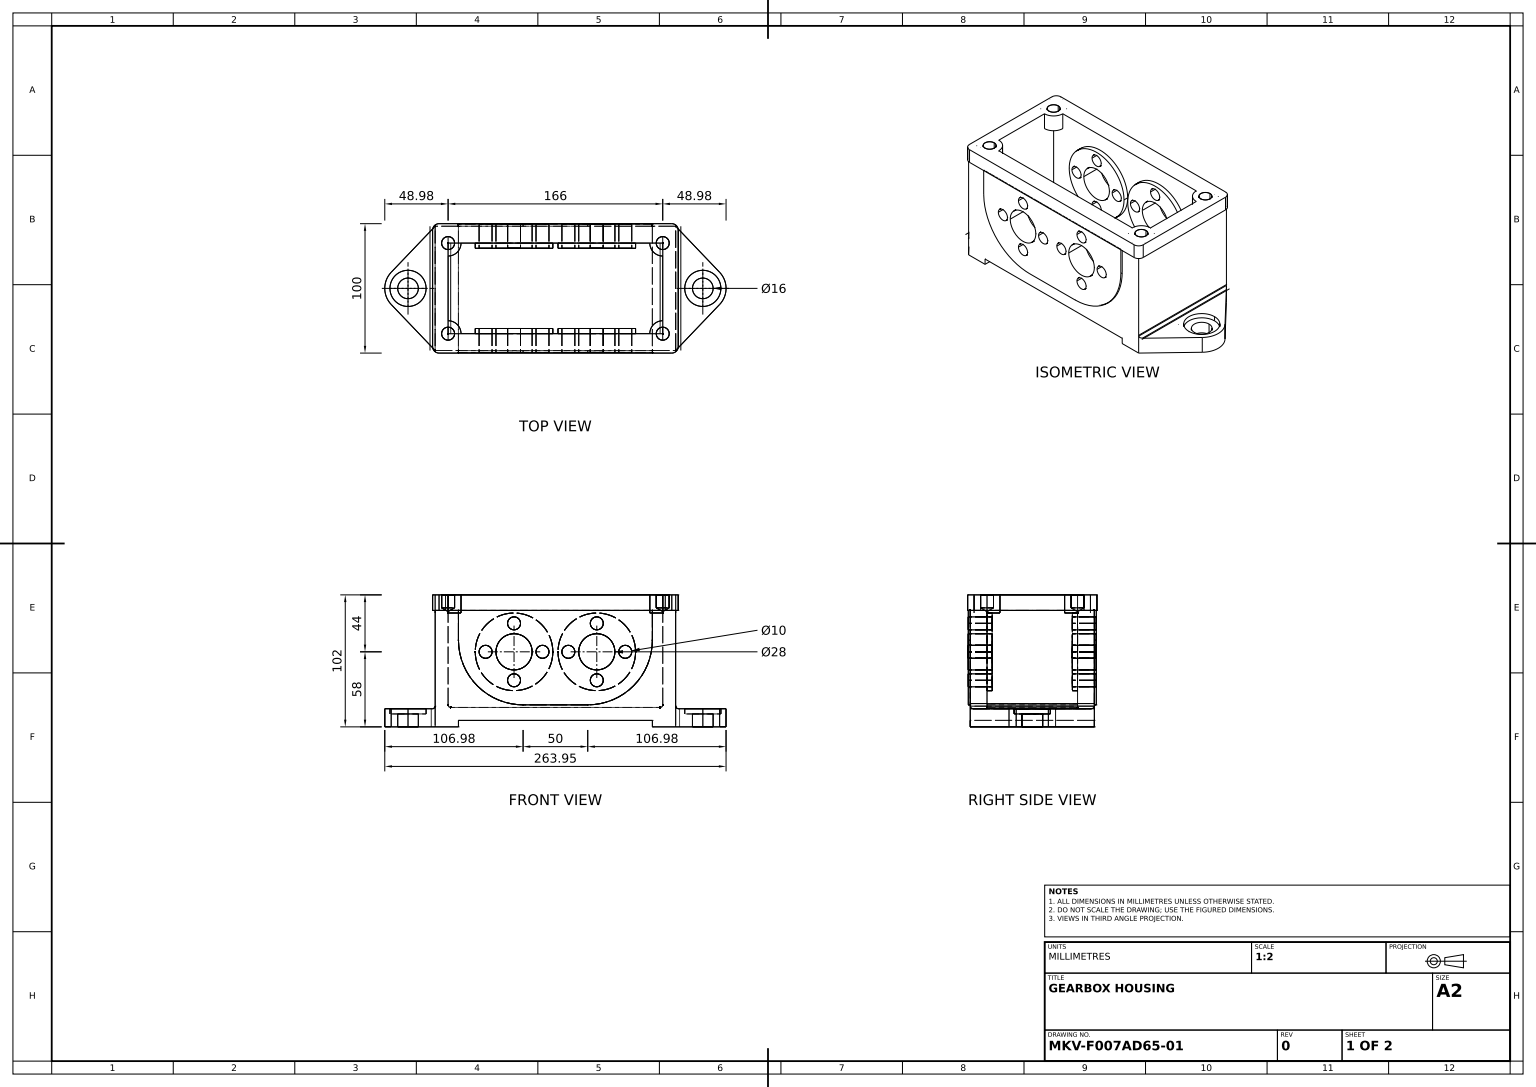
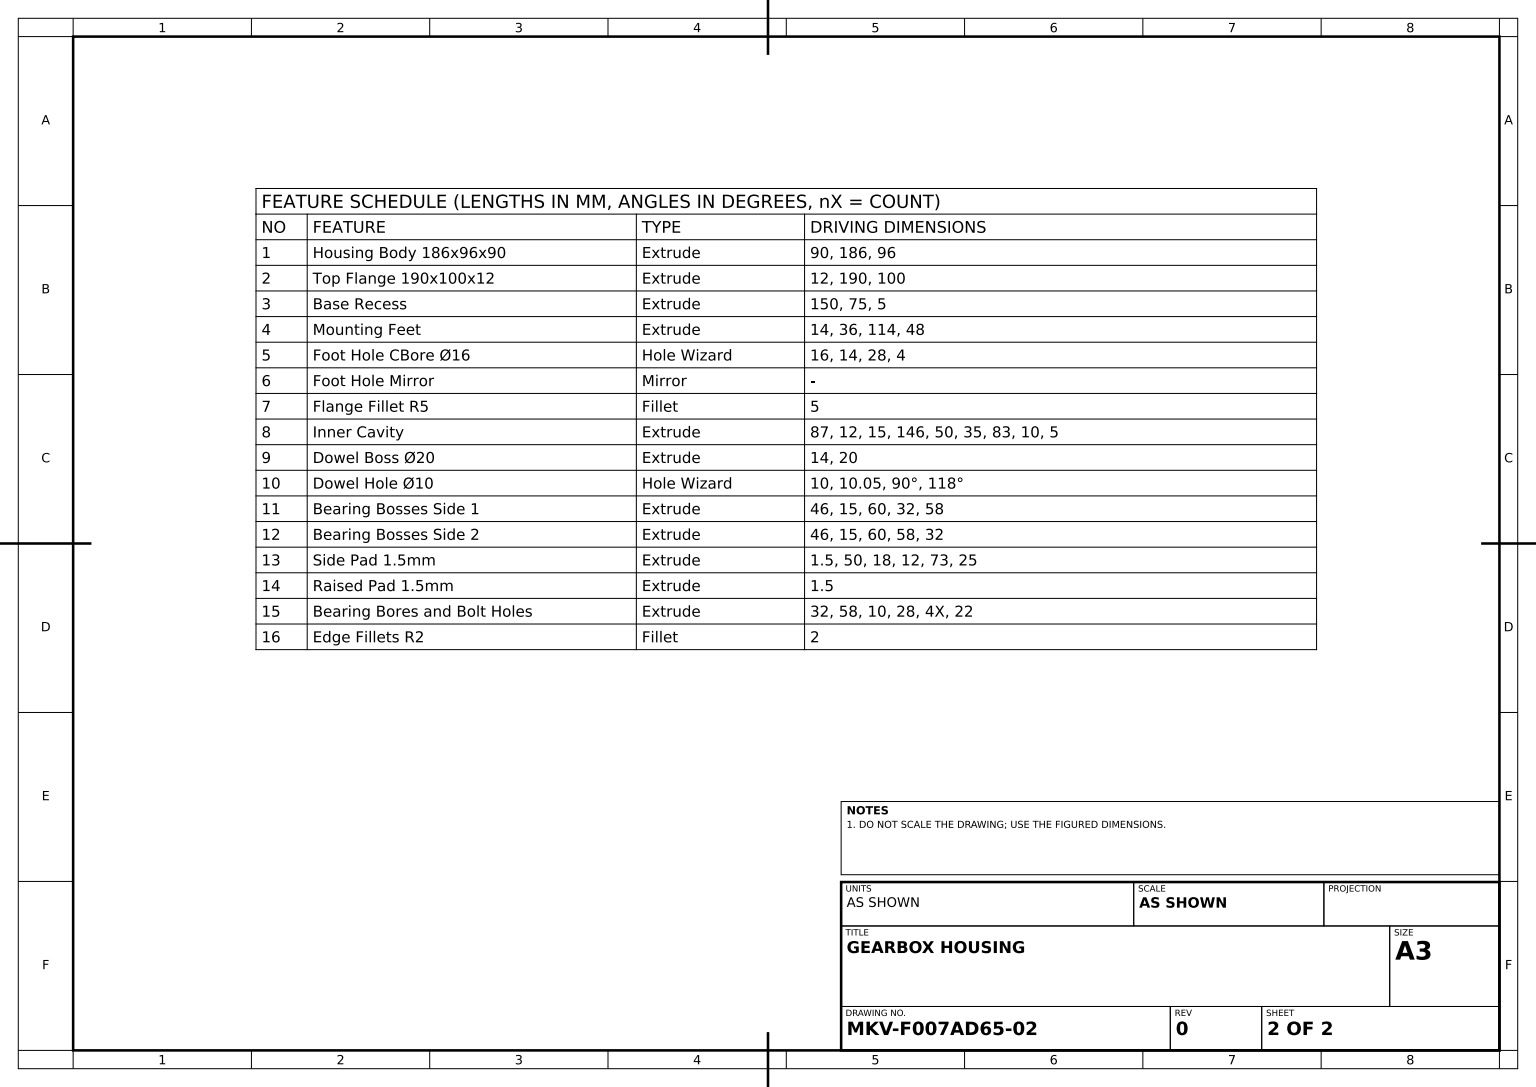
SolidWorks part; units mm, degrees
material "Plain Carbon Steel"
ref_plane "Front Plane" through (0, 0, 0) normal (0, 0, 1) x (1, 0, 0)
ref_plane "Top Plane" through (0, 0, 0) normal (0, 1, 0) x (1, 0, 0)
ref_plane "Right Plane" through (0, 0, 0) normal (1, 0, 0) x (0, 0, -1)
sketch "Housing Body Sketch" plane through (0, 0, 0) normal (0, 1, 0) x (1, 0, 0)
  line L1 (-93, -48) -> (93, -48)
  line L2 (-93, -48) -> (-93, 48)
  line L3 (-93, 48) -> (93, 48)
  line L4 (93, -48) -> (93, 48)
  line L5 (-93, -48) -> (93, 48) construction
  line L6 (-93, 48) -> (93, -48) construction
  point P0 (0, 0)
  dimension "D1" = 186
  dimension "D2" = 96
extrude "Housing Body 186x96x90" add sketch "Housing Body Sketch" along normal blind 90
sketch "Top Flange Sketch" plane through (0, 90, 0) normal (0, 1, 0) x (1, 0, 0)
  line L1 (-95, -50) -> (95, -50)
  line L2 (-95, -50) -> (-95, 50)
  line L3 (-95, 50) -> (95, 50)
  line L4 (95, -50) -> (95, 50)
  line L5 (-95, -50) -> (95, 50) construction
  line L6 (-95, 50) -> (95, -50) construction
  point P0 (0, 0)
  dimension "D1" = 190
  dimension "D2" = 100
extrude "Top Flange 190x100x12" add sketch "Top Flange Sketch" along normal blind 12
sketch "Base Recess Sketch" plane through (0, 0, 48) normal (0, 0, 1) x (1, 0, 0)
  line L0 (-93, 0) -> (93, 0) construction
  line L1 (-75, 0) -> (75, 0)
  line L2 (-75, 0) -> (-75, 5)
  line L3 (-75, 5) -> (75, 5)
  line L4 (75, 0) -> (75, 5)
  dimension "D1" = 150
  dimension "D2" = 75
  dimension "D3" = 5
extrude "Base Recess" cut sketch "Base Recess Sketch" against normal through all
sketch "Mounting Feet Sketch" plane through (0, 0, 0) normal (0, -1, 0) x (1, 0, 0)
  line L0 (75, -48) -> (-75, -48) construction
  line L1 (-127.0084, 12.4412) -> (-93, 48)
  line L2 (-127.0084, -12.4412) -> (-93, -48)
  line L3 (-93, 48) -> (-93, -48)
  arc A0 (-127.0084, 12.4412) -> (-127.0084, -12.4412) centre (-114, 0) ccw
  dimension "D1" = 36
  dimension "D2" = 114
  dimension "D3" = 48
extrude "Mounting Feet" add sketch "Mounting Feet Sketch" against normal blind 14
hole_wizard "Foot Hole CBore Ø16" positions "Sketch5" profile "Sketch6" legacy
sketch "Sketch5" plane through (0, 14, 0) normal (0, 1, 0) x (1, 0, 0)
  point P0 (-114, 0)
sketch "Sketch6" plane through (-114, 14, 0) normal (1, 0, 0) x (0, 0, 1)
  line L0 (0, 0) -> (0, 14)
  line L1 (0, 14) -> (8, 14)
  line L2 (8, 14) -> (8, 4)
  line L3 (8, 4) -> (14, 4)
  line L4 (14, 4) -> (14, 0)
  line L5 (14, 0) -> (0, 0)
  line L6 (0, 110) -> (0, -10) construction
  dimension "Diameter" = 16
  dimension "Depth" = 14
  dimension "C-Bore Diameter" = 28
  dimension "C-Bore Depth" = 4
mirror "Foot Hole Mirror" about plane through (0, 0, 0) normal (1, 0, 0) of "Foot Hole CBore Ø16", "Mounting Feet"
fillet "Flange Fillet R5" radius 5 4 edges at (95, 96, -50) (-95, 96, -50) (95, 96, 50) (-95, 96, 50)
sketch "Inner Cavity Sketch" plane through (0, 102, 0) normal (0, 1, 0) x (1, 0, 0)
  line L0 (-95, 45) -> (-95, -45) construction
  line L1 (-90, -50) -> (90, -50) construction
  line L2 (90, 50) -> (-90, 50) construction
  line L3 (95, -45) -> (95, 45) construction
  line L4 (-73, 35) -> (73, 35)
  line L5 (-73, -35) -> (73, -35)
  line L6 (83, 25) -> (83, -25)
  line L7 (-83, 25) -> (-83, -25)
  line L8 (-83, 25) -> (-83, 35)
  line L9 (-83, 35) -> (-73, 35)
  line L10 (-83, -25) -> (-83, -35)
  line L11 (-83, -35) -> (-73, -35)
  line L12 (83, -25) -> (83, -35)
  line L13 (83, -35) -> (73, -35)
  line L14 (73, 35) -> (83, 35)
  line L15 (83, 35) -> (83, 25)
  point P5 (83, 30)
  dimension "D10" = 35
  dimension "D2" = 12
  dimension "D3" = 15
  dimension "D4" = 12
  dimension "D5" = 15
  dimension "D6" = 15
  dimension "D7" = 12
  dimension "D8" = 12
  dimension "D9" = 15
  dimension "D11" = 146
  dimension "D12" = 50
  dimension "D13" = 35
  dimension "D14" = 83
  dimension "D15" = 83
  dimension "D16" = 10
  dimension "D17" = 5
  dimension "D18" = 10
  dimension "D19" = 10
extrude "Inner Cavity" cut sketch "Inner Cavity Sketch" against normal blind 87
sketch "Dowel Boss Sketch" plane through (0, 102, 0) normal (0, 1, 0) x (1, 0, 0)
  circle A0 centre (-83, 35) radius 10
  circle A1 centre (83, 35) radius 10
  circle A2 centre (83, -35) radius 10
  circle A3 centre (-83, -35) radius 10
  dimension "D1" = 20
extrude "Dowel Boss Ø20" add sketch "Dowel Boss Sketch" against normal blind 14
hole_wizard "Dowel Hole Ø10" positions "Sketch13" profile "Sketch14" hole size "Ø10.0" standard "ISO"
sketch "Sketch13" plane through (0, 102, 0) normal (0, 1, 0) x (1, 0, 0)
  point P0 (-83, -35)
  point P3 (-83, 35)
  point P6 (83, 35)
  point P9 (83, -35)
sketch "Sketch14" plane through (-83, 102, 35) normal (1, 0, 0) x (0, 0, 1)
  line L0 (0, 0) -> (0, 13.0043)
  line L1 (0, 13.0043) -> (5, 10)
  line L2 (5, 10) -> (5, 0.025)
  line L3 (5, 0.025) -> (5.025, 0)
  line L5 (5.025, 0) -> (0, 0)
  line L6 (-5, 0.025) -> (-5.025, 0) construction
  line L10 (0, 13.0043) -> (-5, 10) construction
  line L11 (0, -6.35) -> (0, 107.95) construction
  dimension "Hole Dia." = 10
  dimension "Hole Depth" = 10
  dimension "Near C'Sink Dia." = 10.05
  dimension "Near C'Sink Angle" = 90
  dimension "Drill Angle" = 118
ref_plane "Plane1" through (0, 0, -46) normal (0, 0, 1) x (1, 0, 0)
sketch "Bearing Bosses Side 1 Sketch" plane through (0, 0, -46) normal (0, 0, 1) x (1, 0, 0)
  circle A0 centre (-32, 58) radius 30
  circle A1 centre (32, 58) radius 30
  dimension "D1" = 60
  dimension "D2" = 32
  dimension "D3" = 58
  dimension "D4" = 32
  dimension "D5" = 58
extrude "Bearing Bosses Side 1" add sketch "Bearing Bosses Side 1 Sketch" along normal blind 15
ref_plane "Plane2" through (0, 0, 46) normal (0, 0, 1) x (1, 0, 0)
sketch "Bearing Bosses Side 2 Sketch" plane through (0, 0, 46) normal (0, 0, 1) x (1, 0, 0)
  circle A0 centre (32, 58) radius 30
  circle A1 centre (-32, 58) radius 30
  dimension "D1" = 60
  dimension "D2" = 58
  dimension "D3" = 32
  dimension "D4" = 32
  dimension "D5" = 58
extrude "Bearing Bosses Side 2" add sketch "Bearing Bosses Side 2 Sketch" against normal blind 15
sketch "Side Pad Sketch" plane through (0, 0, -48) normal (0, 0, -1) x (-1, 0, 0)
  line L0 (-93, 90) -> (-93, 14) construction
  line L1 (-25, 17) -> (0, 17)
  line L2 (-75, 90) -> (75, 90)
  line L3 (-75, 90) -> (-75, 67)
  line L4 (0, 17) -> (25, 17)
  line L5 (93, 90) -> (93, 14) construction
  line L6 (75, 90) -> (75, 67)
  line L7 (-75, 5) -> (75, 5) construction
  arc A4 (-75, 67) -> (-25, 17) centre (-25, 67) ccw
  arc A5 (25, 17) -> (75, 67) centre (25, 67) ccw
  dimension "D1" = 18
  dimension "D2" = 50
  dimension "D3" = 18
  dimension "D4" = 12
  dimension "D5" = 73
  dimension "D6" = 25
extrude "Side Pad 1.5mm" add sketch "Side Pad Sketch" along normal blind 1.5
sketch "Raised Pad Sketch" plane through (0, 0, 48) normal (0, 0, 1) x (1, 0, 0)
  line L0 (75, 90) -> (75, 67) construction
  line L1 (25, 17) -> (-25, 17) construction
  line L2 (-75, 67) -> (-75, 90) construction
  line L3 (75, 90) -> (75, 67)
  line L4 (25, 17) -> (-25, 17)
  line L5 (-75, 67) -> (-75, 90)
  line L6 (-75, 90) -> (75, 90)
  arc A0 (25, 17) -> (75, 67) centre (25, 67) ccw construction
  arc A1 (-75, 67) -> (-25, 17) centre (-25, 67) ccw construction
  arc A2 (25, 17) -> (75, 67) centre (25, 67) ccw
  arc A3 (-75, 67) -> (-25, 17) centre (-25, 67) ccw
extrude "Raised Pad 1.5mm" add sketch "Raised Pad Sketch" along normal blind 1.5
sketch "Bearing Bores and Bolt Holes Sketch" plane through (0, 0, 49.5) normal (0, 0, 1) x (1, 0, 0)
  circle A6 centre (-32, 80) radius 5
  circle A7 centre (32, 80) radius 5
  circle A8 centre (-32, 58) radius 14
  circle A9 centre (32, 58) radius 14
  circle A10 centre (-10, 58) radius 5
  circle A11 centre (-32, 36) radius 5
  circle A12 centre (-54, 58) radius 5
  circle A13 centre (54, 58) radius 5
  circle A14 centre (32, 36) radius 5
  circle A15 centre (10, 58) radius 5
  dimension "D1" = 22
  dimension "D2" = 32
  dimension "D6" = 10
  dimension "D7" = 28
  dimension "D3" = 58
  dimension "D4" = 58
  dimension "D5" = 32
  dimension "D10" = 22
  dimension "D11" = 22
  dimension "D12" = 22
  dimension "D13" = 22
  dimension "D14" = 22
  dimension "D8" = 4
  dimension "D9" = 4
extrude "Bearing Bores and Bolt Holes" cut sketch "Bearing Bores and Bolt Holes Sketch" against normal through all
fillet "Edge Fillets R2" radius 2 4 edges at (-93, 14, 0) (93, 14, 0) (83, 15, 0) (-83, 15, 0)
